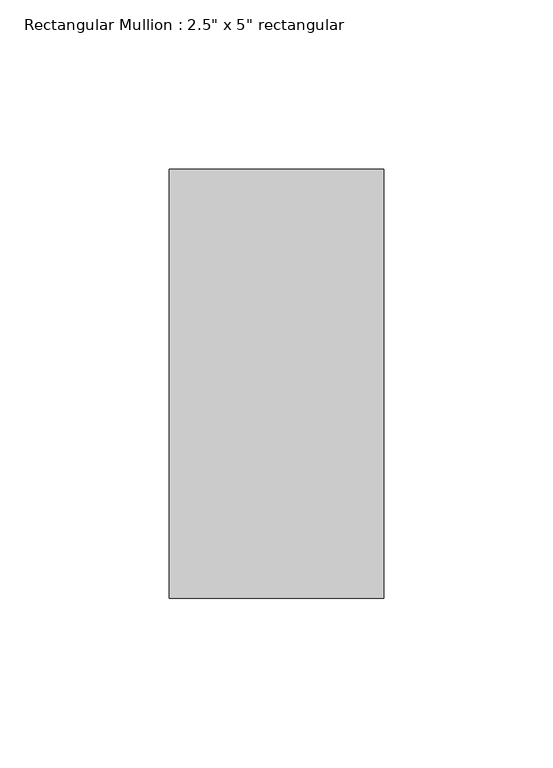
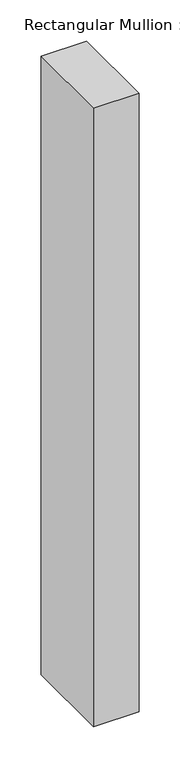
"""IFC4 building model written with IfcOpenShell, lengths in millimetres: member geometry."""

from ifc_helpers import new_model, si_unit, frame, origin, place, context, project, spatial, polyline, outline, extrude, source, transform, mapped, element, save


def member_275f0c90(model_context):
    return source(origin(), model_context, "Body", "SweptSolid", [
        extrude(outline(polyline([(31.75, 63.5), (31.75, -63.5), (-31.75, -63.5), (-31.75, 63.5), (31.75, 63.5)])), frame((0.0, 0.0, -913.799557), z_axis=(0.0, 0.0, 1.0), x_axis=(1.0, 0.0, 0.0)), (0.0, 0.0, 1.0), 913.799557),
    ])


if __name__ == "__main__":
    model = new_model("IFC4")
    model_context = context("Model", 3, world=origin())
    ifc_project = project(units=[si_unit("LENGTHUNIT", "METRE", prefix="MILLI")], contexts=[model_context])
    site = spatial("IfcSite", under=ifc_project)
    building = spatial("IfcBuilding", under=site)
    placement = place(None, origin())
    member_shape = member_275f0c90(model_context)
    element("IfcMember", 1, ObjectType="Rectangular Mullion : 2.5\" x 5\" rectangular", at=placement, inside=building, context=model_context, shape_type="MappedRepresentation", body=[
        mapped(member_shape, transform((0.0, 0.0, 0.0), x_axis=(1.0, 0.0, 0.0), y_axis=(0.0, 1.0, 0.0), z_axis=(0.0, 0.0, 1.0))),
    ])
    save(model, "model.ifc")

# Revit data of these elements
# Type "Rectangular Mullion : 2.5\" x 5\" rectangular"
#   built-in parameter 1007304 = 0.416667 (stored number, unit not read)
#   built-in parameter 1007301 = 0.104167 (stored number, unit not read)
#   built-in parameter 1007300 = 0.104167 (stored number, unit not read)
# Element 1 (IfcMember, "Rectangular Mullion : 2.5\" x 5\" rectangular")
#   Materials on its faces: "Aluminum"
# Materials
#   "Aluminum": class "Metal", colour RGB 247 247 247, transparency 0, Description = "Aluminum 6061", Cost = 0
